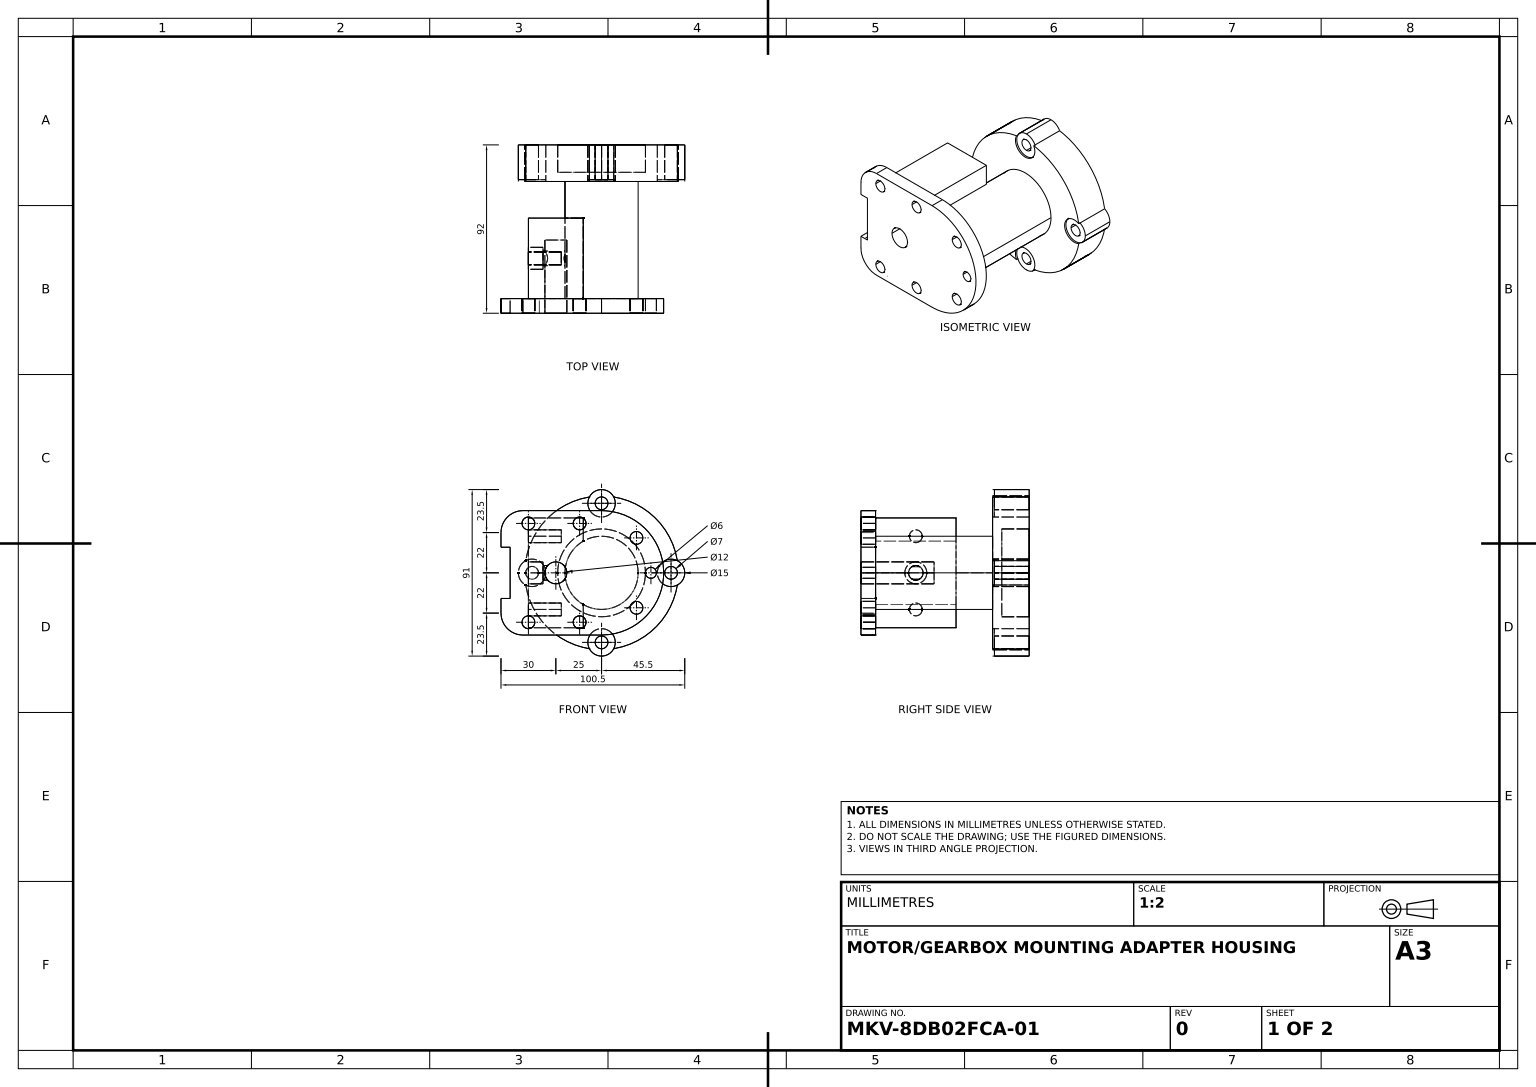
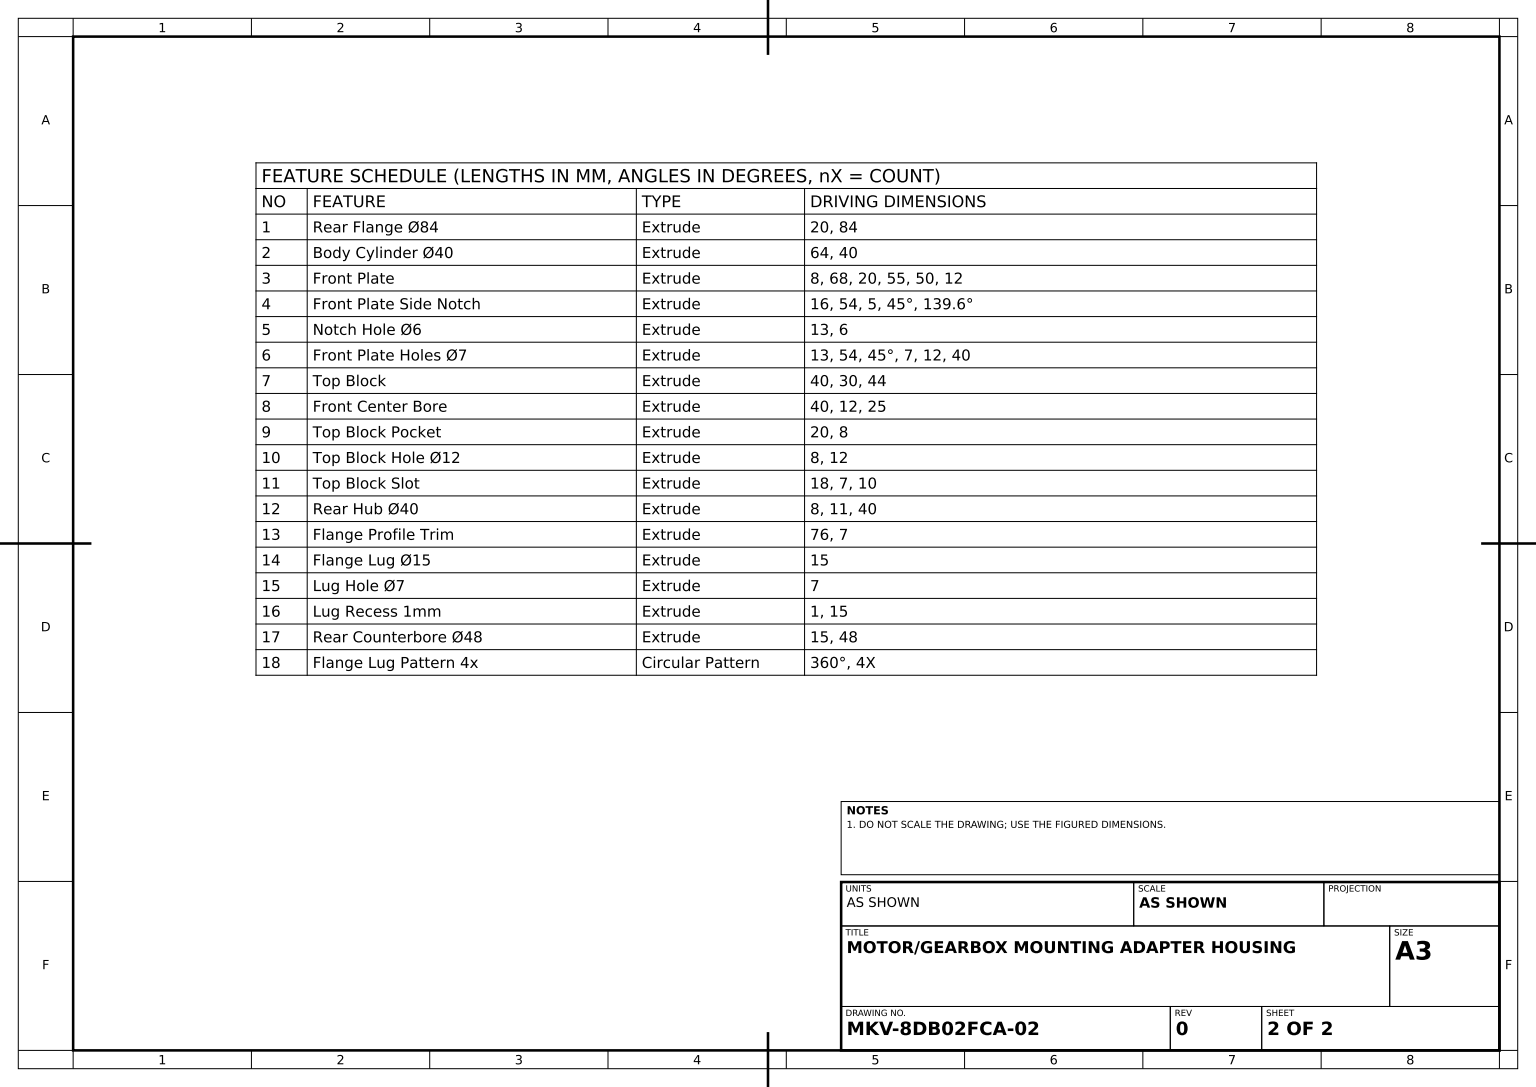
SolidWorks part; units mm, degrees
material "Plain Carbon Steel"
ref_plane "Front Plane" through (0, 0, 0) normal (0, 0, 1) x (1, 0, 0)
ref_plane "Top Plane" through (0, 0, 0) normal (0, 1, 0) x (1, 0, 0)
ref_plane "Right Plane" through (0, 0, 0) normal (1, 0, 0) x (0, 0, -1)
sketch "Rear Flange Sketch Ø84" plane through (0, 0, 0) normal (0, 0, 1) x (1, 0, 0)
  circle A0 centre (0, 0) radius 42
  dimension "D1" = 84
extrude "Rear Flange Ø84" add sketch "Rear Flange Sketch Ø84" along normal blind 20
sketch "Body Cylinder Sketch Ø40" plane through (0, 0, 20) normal (0, 0, 1) x (1, 0, 0)
  circle A0 centre (0, 0) radius 20
  dimension "D1" = 40
extrude "Body Cylinder Ø40" add sketch "Body Cylinder Sketch Ø40" along normal blind 64
sketch "Front Plate Sketch" plane through (0, 0, 84) normal (0, 0, 1) x (1, 0, 0)
  line L0 (0, 0) -> (0, 34) construction
  line L1 (0, 0) -> (0, -34) construction
  line L2 (0, 34) -> (-43, 34)
  line L3 (0, -34) -> (-43, -34)
  line L4 (-55, -22) -> (-55, -14)
  line L6 (-50, 0) -> (-50, 14)
  line L7 (-50, 0) -> (-50, -14)
  line L8 (-50, -14) -> (-55, -14)
  line L9 (-50, 14) -> (-55, 14)
  line L10 (-55, 14) -> (-55, 22)
  arc A0 (0, -34) -> (0, 34) centre (0, 0) ccw
  arc A1 (-43, -34) -> (-55, -22) centre (-43, -22) cw
  arc A2 (-43, 34) -> (-55, 22) centre (-43, 22) ccw
  point P14 (-55, -34)
  point P17 (-55, 34)
  dimension "D1" = 68
  dimension "D6" = 12
  dimension "D2" = 20
  dimension "D3" = 20
  dimension "D4" = 55
  dimension "D5" = 50
extrude "Front Plate" add sketch "Front Plate Sketch" along normal blind 8
sketch "Front Plate Side Notch Sketch" plane through (0, 0, 92) normal (0, 0, 1) x (1, 0, 0)
  line L2 (0, 0) -> (27, 0) construction
  line L3 (0, 0) -> (19.0919, 19.0919) construction
  line L4 (0, 0) -> (20.5513, -17.5113) construction
  circle A0 centre (0, 0) radius 27 construction
  circle A1 centre (27, 0) radius 2.5
  dimension "D1" = 54
  dimension "D2" = 5
  dimension "D3" = 45
  dimension "D4" = 139.566
extrude "Front Plate Side Notch" cut sketch "Front Plate Side Notch Sketch" against normal blind 16
sketch "Notch Hole Sketch Ø6" plane through (0, 0, 92) normal (0, 0, 1) x (1, 0, 0)
  circle A0 centre (27, 0) radius 3
  dimension "D1" = 6
extrude "Notch Hole Ø6" cut sketch "Notch Hole Sketch Ø6" against normal blind 13
sketch "Front Plate Holes Sketch" plane through (0, 0, 92) normal (0, 0, 1) x (1, 0, 0)
  line L0 (0, 27) -> (-58.7136, 27) construction
  line L1 (0, -27) -> (-58.7136, -27) construction
  line L2 (0, 0) -> (19.0919, 19.0919) construction
  line L3 (0, 0) -> (19.0919, -19.0919) construction
  line L4 (0, 0) -> (27, 0) construction
  line L5 (0, 27) -> (-12, 27) construction
  line L6 (-12, 27) -> (-40, 27) construction
  line L7 (0, -27) -> (-12, -27) construction
  line L8 (-12, -27) -> (-40, -27) construction
  circle A0 centre (0, 0) radius 27 construction
  circle A1 centre (19.0919, 19.0919) radius 3.5
  circle A2 centre (19.0919, -19.0919) radius 3.5
  circle A3 centre (-12, 27) radius 3.5
  circle A4 centre (-40, 27) radius 3.5
  circle A5 centre (-12, -27) radius 3.5
  circle A6 centre (-40, -27) radius 3.5
  dimension "D1" = 54
  dimension "D2" = 45
  dimension "D4" = 7
  dimension "D5" = 7
  dimension "D6" = 7
  dimension "D7" = 7
  dimension "D10" = 7
  dimension "D11" = 7
  dimension "D3" = 45
  dimension "D8" = 12
  dimension "D9" = 40
  dimension "D12" = 12
  dimension "D13" = 40
extrude "Front Plate Holes Ø7" cut sketch "Front Plate Holes Sketch" against normal blind 13
ref_plane "Top Block Plane" through (-40, 0, 0) normal (1, 0, 0) x (0, 0, -1)
sketch "Top Block Sketch" plane through (-40, 0, 0) normal (1, 0, 0) x (0, 0, -1)
  line L9 (-84, 0) -> (-84, -30.5)
  line L10 (-84, -30) -> (-40, -30)
  line L11 (-84, -34) -> (-84, 34) construction
  line L12 (-40, -30) -> (-40, 0)
  line L14 (-84, 0) -> (-84, 30)
  line L15 (-84, 30) -> (-40, 30)
  line L16 (-40, 30) -> (-40, 0)
  dimension "D1" = 44
  dimension "D2" = 30
extrude "Top Block" add sketch "Top Block Sketch" along normal blind 30 contours L16 L15 L14 L9 L10 L12
sketch "Front Center Bore Sketch" plane through (0, 0, 92) normal (0, 0, 1) x (1, 0, 0)
  line L0 (0, 0) -> (-25, 0) construction
  circle A1 centre (-25, 0) radius 6
  dimension "D1" = 12
  dimension "D2" = 25
extrude "Front Center Bore" cut sketch "Front Center Bore Sketch" against normal blind 40
sketch "Top Block Pocket Sketch" plane through (-40, 0, 0) normal (-1, 0, 0) x (0, 0, 1)
  line L0 (84, 0) -> (40, 0) construction
  line L3 (84, -23.5) -> (84, 23.5) construction
  line L4 (40, 30) -> (40, -30) construction
  circle A0 centre (62, 0) radius 4
  dimension "D1" = 8
extrude "Top Block Pocket" cut sketch "Top Block Pocket Sketch" against normal blind 20
sketch "Top Block Hole Sketch Ø12" plane through (-40, 0, 0) normal (-1, 0, 0) x (0, 0, 1)
  circle A0 centre (62, 0) radius 6
  dimension "D1" = 12
extrude "Top Block Hole Ø12" cut sketch "Top Block Hole Sketch Ø12" against normal blind 8
sketch "Top Block Slot Sketch" plane through (-40, 0, 0) normal (-1, 0, 0) x (0, 0, 1)
  line L0 (62, 0) -> (62, 20) construction
  line L1 (62, 0) -> (62, -20) construction
  line L2 (84, -30) -> (40, -30) construction
  circle A0 centre (62, 20) radius 3.5
  circle A1 centre (62, -20) radius 3.5
  dimension "D1" = 7
  dimension "D2" = 10
extrude "Top Block Slot" cut sketch "Top Block Slot Sketch" against normal blind 18
ref_plane "Rear Hub Plane" through (0, 0, 8) normal (0, 0, 1) x (1, 0, 0)
sketch "Rear Hub Sketch Ø40" plane through (0, 0, 8) normal (0, 0, 1) x (1, 0, 0)
  circle A0 centre (0, 0) radius 20
  dimension "D1" = 40
extrude "Rear Hub Ø40" add sketch "Rear Hub Sketch Ø40" along normal blind 11
sketch "Flange Profile Trim Sketch" plane through (0, 0, 20) normal (0, 0, 1) x (1, 0, 0)
  line L0 (0, 0) -> (38, 0) construction
  circle A0 centre (0, 0) radius 38 construction
  circle A1 centre (38, 0) radius 3.5
  dimension "D1" = 76
  dimension "D2" = 7
extrude "Flange Profile Trim" cut sketch "Flange Profile Trim Sketch" against normal through all
sketch "Flange Lug Sketch Ø15" plane through (0, 0, 20) normal (0, 0, 1) x (1, 0, 0)
  circle A0 centre (38, 0) radius 7.5
  dimension "D1" = 15
extrude "Flange Lug Ø15" add sketch "Flange Lug Sketch Ø15" against normal through all
sketch "Lug Hole Sketch Ø7" plane through (0, 0, 20) normal (0, 0, 1) x (1, 0, 0)
  circle A0 centre (38, 0) radius 3.5
  dimension "D1" = 7
extrude "Lug Hole Ø7" cut sketch "Lug Hole Sketch Ø7" against normal through all
sketch "Lug Recess Sketch" plane through (0, 0, 20) normal (0, 0, 1) x (1, 0, 0)
  circle A0 centre (38, 0) radius 7.5
  dimension "D1" = 15
extrude "Lug Recess 1mm" cut sketch "Lug Recess Sketch" against normal blind 1
sketch "Rear Counterbore Sketch Ø48" plane through (0, 0, 0) normal (0, 0, -1) x (-1, 0, 0)
  circle A0 centre (0, 0) radius 24
  dimension "D1" = 48
extrude "Rear Counterbore Ø48" cut sketch "Rear Counterbore Sketch Ø48" against normal blind 15
pattern_circular "Flange Lug Pattern 4x" count 4 over 360 about axis through (0, 0, 0) along (0, 0, 1) of "Lug Recess 1mm", "Lug Hole Ø7", "Flange Lug Ø15"
